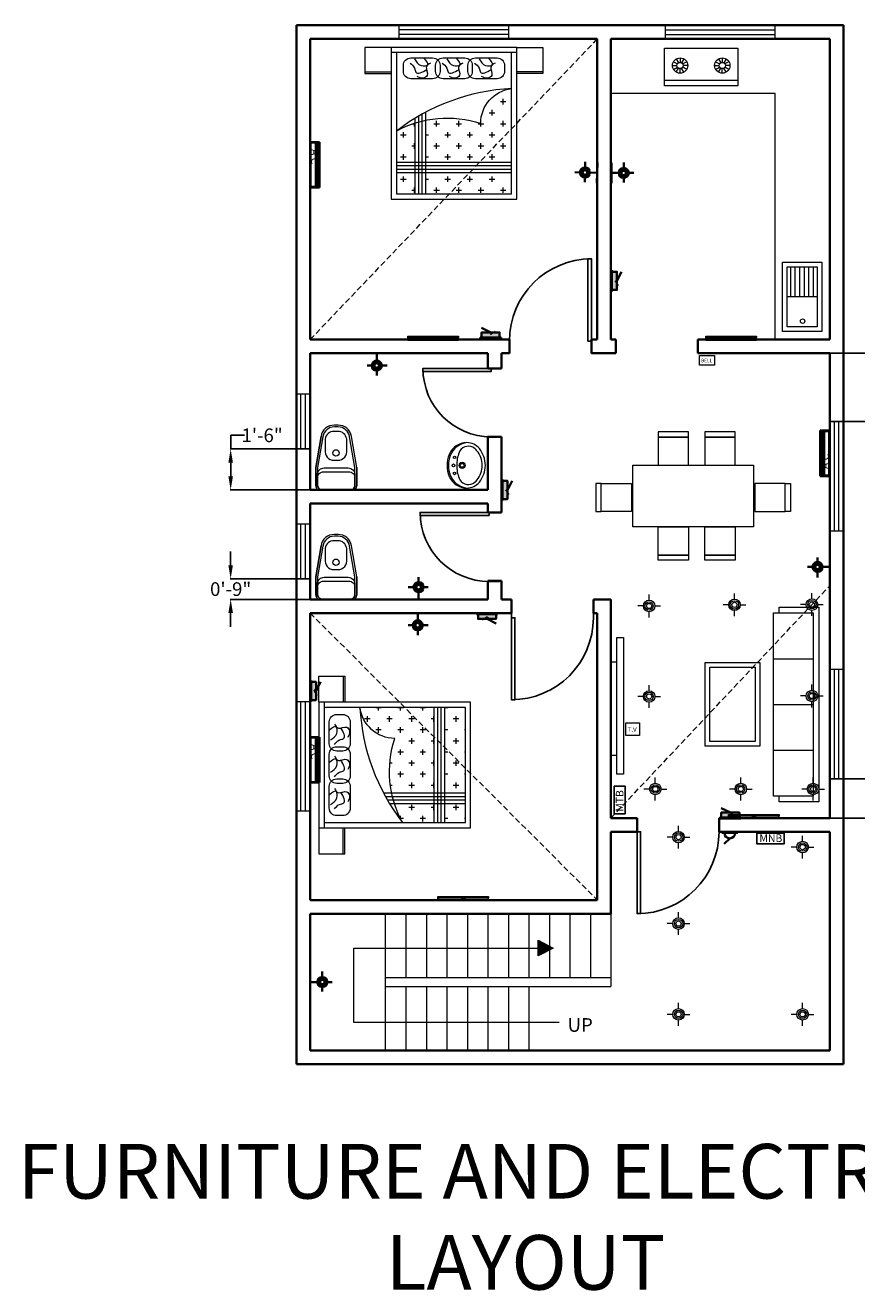
# Model space of a CAD drawing. Units: inches. Extents: x 329 to 1300, y 173 to 760.
# Tile 2 of 3: x 720 to 1085, y 173 to 729. Entities that reach past the tile are written whole.
import ezdxf

# ---------------------------------------------------------------- set-up
doc = ezdxf.new("R2010")
doc.units = ezdxf.units.IN
doc.header["$MEASUREMENT"] = 0
doc.linetypes.add('HIDDEN', pattern=[0.375, 0.25, -0.125])
for name, color, linetype, lineweight in [('A -Elec', 6, 'Continuous', 18), ('A-ANNO-SYMB', 7, 'Continuous', 18), ('A-ANNO-TEXT', 7, 'Continuous', 18), ('A-ANNO-TITL', 1, 'Continuous', 25), ('A-EQPM', 8, 'Continuous', 18), ('A-FLOR-CASE', 163, 'Continuous', 18), ('A-FLOR-FIXT', 163, 'Continuous', 18), ('A-FLOR-STRS', 7, 'Continuous', 18), ('A-FURN', 150, 'Continuous', 5), ('A-GLAZ', 4, 'Continuous', 18), ('A-WALL', 7, 'Continuous', 35), ('DIMENSION', 80, 'Continuous', 13), ('DOOR', 27, 'Continuous', 25), ('E-COMM', 1, 'Continuous', 18), ('E-EQPM-HIDN', 1, 'HIDDEN', 13), ('E-LITE', 6, 'Continuous', 18), ('E-LITE-SWCH', 1, 'Continuous', 18), ('E-POWR-PANL', 1, 'Continuous', 25), ('Elec', 1, 'Continuous', 35), ('FURN', 163, 'Continuous', 5), ('FURNITURE', 163, 'Continuous', 18), ('M-HVAC-EQPM', 1, 'Continuous', 18)]:
    doc.layers.add(name, color=color, linetype=linetype, lineweight=lineweight)
doc.layers.add('A-ANNO-PATT', color=251, linetype='Continuous', lineweight=13, true_color=0x636466)
doc.styles.get("Standard").update_dxf_attribs({"font": 'arial.ttf'})
doc.dimstyles.get("Standard").update_dxf_attribs({"dimtxt": 6, "dimasz": 6, "dimexe": 0.18, "dimexo": 0.0625, "dimgap": 0.09, "dimtad": 0, "dimtih": 1, "dimtoh": 1, "dimdec": 1, "dimzin": 0, "dimdsep": 46, "dimlunit": 3, "dimtxsty": 'Standard', "dimcen": 0.09, "dimadec": 0, "dimazin": 0, "dimtfac": 1, "dimtdec": 1, "dimtofl": 0, "dimtmove": 0, "dimatfit": 3, "dimfxl": 1, "dimtolj": 1, "dimtzin": 0, "dimarcsym": 0})

# ---------------------------------------------------------------- blocks, each defined once
blk = doc.blocks.new('*U2')
for p, q in [((0, 0), (0, -6)), ((40, 0), (40, -6))]:
    blk.add_line(p, q)
blk.add_lwpolyline([(0, 0), (0, 40), (1.75, 40), (1.75, 0)], close=True)
blk.add_arc((0, 0), 40, 0, 90)
blk = doc.blocks.new('TV')
for points in [[(1846.64, 1133.16), (1849.49, 1133.16), (1849.49, 1073.14), (1846.64, 1073.14)], [(1846.64, 1122.37), (1844, 1122.37), (1844, 1081.48), (1846.64, 1081.48)]]:
    blk.add_lwpolyline(points, close=True)
blk = doc.blocks.new('SINK')
for p, q in [((1691.4, 1155.42), (1708.6, 1155.42)), ((1708.6, 1155.42), (1708.6, 1125.07)), ((1693.4, 1140.25), (1706.6, 1140.25)), ((1695.01, 1140.25), (1695.01, 1127.07)), ((1697.01, 1140.25), (1697.01, 1127.07)), ((1699.01, 1140.25), (1699.01, 1127.07)), ((1701.01, 1140.25), (1701.01, 1127.07)), ((1703.01, 1140.25), (1703.01, 1127.07)), ((1705.01, 1140.25), (1705.01, 1127.07))]:
    blk.add_line(p, q)
for points in [[(1691.4, 1155.42), (1708.6, 1155.42), (1708.6, 1125.07), (1691.4, 1125.07)], [(1693.4, 1153.42), (1706.6, 1153.42), (1706.6, 1127.07), (1693.4, 1127.07)]]:
    blk.add_lwpolyline(points, close=True)
blk.add_circle((1699.78, 1150.93), 0.965)
blk = doc.blocks.new('*U16')
blk.add_line((0, 1), (0, -1))
blk = doc.blocks.new('*U17')
at = {"layer": 'FURN', "transparency": 16777216}
for p, rotation in [((1739.06, 1057.24), 90), ((1739.38, 1058.42), 59.99999999999999), ((1739.38, 1056.06), 120), ((1740.24, 1059.29), 30), ((1740.24, 1055.19), 150), ((1741.42, 1054.87), 180), ((1742.61, 1059.29), 330.0000000000001), ((1742.61, 1055.19), 210), ((1743.47, 1058.42), 300), ((1743.47, 1056.06), 240), ((1743.79, 1057.24), 270)]:
    blk.add_blockref('*U16', p, dxfattribs=dict(at, rotation=rotation))
blk.add_blockref('*U16', (1741.42, 1059.61), dxfattribs=at)
blk = doc.blocks.new('*U18')
blk.add_line((0, 1), (0, -1))
blk = doc.blocks.new('*U19')
at = {"layer": 'FURN', "transparency": 16777216}
for p, rotation in [((1739.06, 1057.24), 90), ((1739.38, 1058.42), 59.99999999999999), ((1739.38, 1056.06), 120), ((1740.24, 1059.29), 30), ((1740.24, 1055.19), 150), ((1741.42, 1054.87), 180), ((1742.61, 1059.29), 330.0000000000001), ((1742.61, 1055.19), 210), ((1743.47, 1058.42), 300), ((1743.47, 1056.06), 240), ((1743.79, 1057.24), 270)]:
    blk.add_blockref('*U18', p, dxfattribs=dict(at, rotation=rotation))
blk.add_blockref('*U18', (1741.42, 1059.61), dxfattribs=at)
blk = doc.blocks.new('GAS')
at = {"layer": 'FURN'}
blk.add_line((1734.58, 1063.74), (1766.85, 1063.74), dxfattribs=at)
blk.add_lwpolyline([(1734.58, 1066.15), (1766.85, 1066.15), (1766.85, 1049.65), (1734.58, 1049.65)], close=True, dxfattribs=at)
for centre, radius in [((1741.42, 1057.24), 3.37), ((1741.42, 1057.24), 1.37), ((1759.93, 1057.24), 3.37), ((1759.93, 1057.24), 1.37)]:
    blk.add_circle(centre, radius, dxfattribs=at)
for name, p in [('*U17', (0, 0)), ('*U19', (18.51, 0))]:
    blk.add_blockref(name, p, dxfattribs=at)
blk = doc.blocks.new('bed 1')
at = {"layer": 'FURN'}
h = blk.add_hatch(dxfattribs=at)
h.set_pattern_fill('CROSS', color=256, style=0)
h.set_pattern_definition([(0, (0, 0), (6.35, 6.35), [3.175, -9.525]), (90, (1.5875, -1.5875), (-6.35, 6.35), [3.175, -9.525])])
h.paths.add_polyline_path([(1334.16, -843.32, 0.37496), (1316.43, -863.27, 0.131129), (1284.95, -861.51), (1284.95, -885.72), (1334.16, -885.72)])
h.paths.add_polyline_path([(1278.95, -863.08, 0.048033), (1268.16, -867.67), (1268.16, -885.72), (1278.95, -885.72)])
h.paths.add_polyline_path([(1278.95, -891.72), (1268.16, -891.72), (1268.16, -903.72), (1278.95, -903.72)])
h.paths.add_polyline_path([(1334.16, -891.72), (1284.95, -891.72), (1284.95, -903.72), (1334.16, -903.72)])
for p, q in [((1265.16, -819.72), (1250.16, -819.72)), ((1250.16, -819.72), (1250.16, -834.72)), ((1337.16, -819.72), (1265.16, -819.72)), ((1265.16, -819.72), (1265.16, -906.72)), ((1337.16, -906.72), (1337.16, -819.72)), ((1337.16, -819.72), (1352.16, -819.72)), ((1352.16, -819.72), (1352.16, -834.72)), ((1337.16, -822.72), (1265.16, -822.72)), ((1268.16, -822.72), (1268.16, -903.72)), ((1334.16, -903.72), (1334.16, -822.72)), ((1250.16, -833.72), (1265.16, -833.72)), ((1352.16, -833.72), (1337.16, -833.72)), ((1250.16, -834.72), (1265.16, -834.72)), ((1352.16, -834.72), (1337.16, -834.72)), ((1278.95, -903.72), (1278.95, -860.29)), ((1280.95, -903.72), (1280.95, -859.11)), ((1282.95, -903.72), (1282.95, -857.98)), ((1284.95, -903.72), (1284.95, -856.89)), ((1334.16, -885.72), (1268.16, -885.72)), ((1334.16, -887.72), (1268.16, -887.72)), ((1334.16, -889.72), (1268.16, -889.72)), ((1334.16, -891.72), (1268.16, -891.72)), ((1265.16, -906.72), (1337.16, -906.72)), ((1268.16, -903.72), (1334.16, -903.72))]:
    blk.add_line(p, q, dxfattribs=at)
for points in [[(1288.91, -837.72), (1276.42, -837.72, -0.414214), (1272.16, -833.47), (1272.16, -829.98, -0.414214), (1276.42, -825.72), (1288.91, -825.72, -0.414214), (1293.16, -829.98), (1293.16, -833.47, -0.414214)], [(1307.41, -837.72), (1294.92, -837.72, -0.414214), (1290.66, -833.47), (1290.66, -829.98, -0.414214), (1294.92, -825.72), (1307.41, -825.72, -0.414214), (1311.66, -829.98), (1311.66, -833.47, -0.414214)], [(1325.91, -837.72), (1313.42, -837.72, -0.414214), (1309.16, -833.47), (1309.16, -829.98, -0.414214), (1313.42, -825.72), (1325.91, -825.72, -0.414214), (1330.16, -829.98), (1330.16, -833.47, -0.414214)], [(1334.16, -843.32, 0.151933), (1268.16, -867.67), (1268.16, -867.67, -0.20661), (1316.43, -863.27), (1316.43, -863.27, -0.37496)]]:
    blk.add_lwpolyline(points, format="xyb", close=True, dxfattribs=at)
for points, knots in [([(1278.62, -826.37), (1279.52, -827.92), (1281.07, -830.61), (1287.77, -830.3), (1285.41, -827.44), (1284.17, -825.93)], [0, 0, 0, 0, 4.23607, 7.317462, 10.761159, 10.761159, 10.761159, 10.761159]), ([(1297.12, -826.37), (1298.02, -827.92), (1299.57, -830.61), (1306.27, -830.3), (1303.91, -827.44), (1302.67, -825.93)], [0, 0, 0, 0, 4.23607, 7.317462, 10.761159, 10.761159, 10.761159, 10.761159]), ([(1315.62, -826.37), (1316.52, -827.92), (1318.07, -830.61), (1324.77, -830.3), (1322.41, -827.44), (1321.17, -825.93)], [0, 0, 0, 0, 4.23607, 7.317462, 10.761159, 10.761159, 10.761159, 10.761159]), ([(1275.98, -828.74), (1277, -829.54), (1278.71, -830.85), (1279.22, -835.95), (1282.92, -833.91), (1285.58, -832.44)], [0, 0, 0, 0, 3.079719, 5.108686, 10.317752, 10.317752, 10.317752, 10.317752]), ([(1287.7, -828.74), (1286.63, -829.38), (1283.96, -830.98), (1287.28, -835.52), (1283.18, -838.02), (1281.17, -836.99), (1280.03, -836.4)], [0, 0, 0, 0, 2.624379, 6.568207, 8.823918, 11.783788, 11.783788, 11.783788, 11.783788]), ([(1294.48, -828.74), (1295.5, -829.54), (1297.21, -830.85), (1297.72, -835.95), (1301.42, -833.91), (1304.08, -832.44)], [0, 0, 0, 0, 3.079719, 5.108686, 10.317752, 10.317752, 10.317752, 10.317752]), ([(1306.2, -828.74), (1305.13, -829.38), (1302.46, -830.98), (1305.78, -835.52), (1301.68, -838.02), (1299.67, -836.99), (1298.53, -836.4)], [0, 0, 0, 0, 2.624379, 6.568207, 8.823918, 11.783788, 11.783788, 11.783788, 11.783788]), ([(1312.98, -828.74), (1314, -829.54), (1315.71, -830.85), (1316.22, -835.95), (1319.92, -833.91), (1322.58, -832.44)], [0, 0, 0, 0, 3.079719, 5.108686, 10.317752, 10.317752, 10.317752, 10.317752]), ([(1324.7, -828.74), (1323.63, -829.38), (1320.96, -830.98), (1324.28, -835.52), (1320.18, -838.02), (1318.17, -836.99), (1317.03, -836.4)], [0, 0, 0, 0, 2.624379, 6.568207, 8.823918, 11.783788, 11.783788, 11.783788, 11.783788])]:
    blk.add_open_spline(points, degree=3, knots=knots, dxfattribs=at)
blk = doc.blocks.new('WC')
at = {"layer": 'A-FURN'}
for p, q in [((171114.18, -56009.21), (171100.52, -56011.54)), ((171114.18, -56009.21), (171122.29, -56009.21)), ((171124.07, -56010.99), (171124.07, -56025.42)), ((171095.59, -56017.39), (171095.59, -56019.02)), ((171114.18, -56027.21), (171100.52, -56024.87)), ((171122.29, -56027.21), (171114.18, -56027.21))]:
    blk.add_line(p, q, dxfattribs=at)
for points in [[(171114.18, -56027.21), (171122.29, -56027.21, 0.414214), (171124.07, -56025.42), (171124.07, -56010.99, 0.414214), (171122.29, -56009.21), (171114.18, -56009.21), (171100.52, -56011.54, 0.365402), (171095.59, -56017.39), (171095.59, -56019.02, 0.365402), (171100.52, -56024.87)], [(171114.25, -56026.41), (171121.5, -56026.41, 0.361508), (171124.07, -56024.7), (171124.07, -56011.71, 0.375474), (171121.68, -56010), (171114.25, -56010), (171100.66, -56012.32, 0.365402), (171096.38, -56017.39), (171096.38, -56019.02, 0.365402), (171100.66, -56024.09)], [(171124.07, -56011.71), (171124.07, -56024.7, -0.361508), (171121.5, -56026.41), (171117.23, -56026.41, -0.430105), (171114.38, -56023.46), (171114.38, -56012.95, -0.411531), (171117.23, -56010), (171121.68, -56010, -0.375474)], [(171124.07, -56011.71), (171124.07, -56024.7, -0.361508), (171121.5, -56026.41), (171118.83, -56026.41, -0.480412), (171116.16, -56023.63), (171116.16, -56012.78, -0.482705), (171118.83, -56010), (171121.68, -56010, -0.375474)], [(171106.42, -56023.02, 0.46477), (171111.04, -56019.12), (171111.04, -56017.49, 0.46477), (171106.42, -56013.59), (171101.64, -56013.59, 0.365402), (171098.35, -56017.49), (171098.35, -56019.12, 0.365402), (171101.64, -56023.02)], [(171107.8, -56016.9, -1), (171107.8, -56019.71, -1)]]:
    blk.add_lwpolyline(points, format="xyb", close=True, dxfattribs=at)
for centre, radius, start, end in [((171122.29, -56010.99), 1.78, 0.0002, 90.0002), ((171101.52, -56017.39), 5.93, 99.7106, 180.0002), ((171101.52, -56019.02), 5.93, 180.0002, 260.2897), ((171122.29, -56025.42), 1.78, 270.0002, 0.0002)]:
    blk.add_arc(centre, radius, start, end, dxfattribs=at)
blk = doc.blocks.new('Basin')
at = {"layer": 'A-FURN'}
for centre, radius in [((171010.96, -56068.51), 0.593), ((171010.45, -56072.47), 0.692), ((171014.68, -56072.47), 1.48), ((171014.68, -56072.47), 0.91), ((171010.96, -56076.42), 0.593)]:
    blk.add_circle(centre, radius, dxfattribs=at)
for centre, radius, start, end in [((171016.96, -56070.69), 9.3, 90, 157.28559), ((171018.29, -56071.51), 10.2, 100.99675, 157.82074), ((171016.96, -56069.3), 7.91, 39.08291, 90), ((171021.21, -56072.47), 13.91, 157.28559, 180), ((171021.21, -56072.47), 13.27, 158.74675, 180), ((171018.29, -56073.43), 10.2, 262.50469, 262.50469), ((171029.84, -56072.47), 17.8, 159.64154, 180), ((171017.65, -56067.95), 4.81, 62.93101, 159.64154), ((171016.96, -56069.3), 6.33, 39.08291, 62.931), ((171013.06, -56072.47), 11.35, 0, 39.08291), ((171013.06, -56072.47), 12.93, 0, 39.08291), ((171021.21, -56072.47), 13.91, 180, 202.71441), ((171021.21, -56072.47), 13.27, 180, 201.25325), ((171029.84, -56072.47), 17.8, 180, 200.35846), ((171013.06, -56072.47), 11.35, 320.91709, 0), ((171013.06, -56072.47), 12.93, 320.91709, 0), ((171016.96, -56074.25), 9.3, 202.71441, 270), ((171018.29, -56073.43), 10.2, 202.17926, 259.00325), ((171017.65, -56076.99), 4.81, 200.35846, 297.06899), ((171016.96, -56075.63), 6.33, 297.069, 320.91709), ((171016.96, -56075.63), 7.91, 270, 320.91709)]:
    blk.add_arc(centre, radius, start, end, dxfattribs=at)
blk = doc.blocks.new('S')
at = {"layer": 'FURN'}
for p, q in [((1046.36, 480.08), (1063.8, 480.08)), ((1046.36, 459.98), (1063.8, 459.98)), ((1046.36, 439.88), (1063.8, 439.88))]:
    blk.add_line(p, q, dxfattribs=at)
blk.add_lwpolyline([(1063.8, 500.18), (1063.8, 419.78), (1046.36, 419.78), (1046.36, 500.18)], close=True, dxfattribs=at)
blk.add_lwpolyline([(1048.87, 500.18), (1048.87, 502.69), (1066.31, 502.69), (1066.31, 417.27), (1048.87, 417.27), (1048.87, 419.78)], dxfattribs=at)
blk = doc.blocks.new('splight')
at = {"layer": 'Elec'}
for p, q in [((4618.17, 527.16), (4627.57, 527.16)), ((4622.87, 527.16), (4622.87, 523.87)), ((4620.58, 521.58), (4618.05, 521.58)), ((4625.16, 521.58), (4627.23, 521.58)), ((4622.87, 519.28), (4622.87, 517.03))]:
    blk.add_line(p, q, dxfattribs=at)
for radius in [2.29, 1.67, 1.04]:
    blk.add_circle((4622.87, 521.58), radius, dxfattribs=at)
blk = doc.blocks.new('tube')
at = {"layer": 'A -Elec'}
for p, q in [((4592.6, 556.8), (4641.6, 556.8)), ((4592.6, 555.3), (4592.6, 556.8)), ((4592.6, 552.8), (4592.6, 555.3)), ((4592.6, 552.8), (4641.6, 552.8)), ((4593.1, 555.3), (4593.1, 556.8)), ((4593.1, 556.3), (4593.4, 556.3)), ((4593.1, 556.2), (4593.4, 556.2)), ((4593.1, 555.8), (4593.4, 555.8)), ((4593.1, 555.7), (4593.4, 555.7)), ((4641.1, 555.3), (4593.1, 555.3)), ((4593.1, 555.3), (4593.1, 553.3)), ((4593.1, 553.3), (4593.1, 555.3)), ((4593.1, 553.3), (4641.6, 553.3)), ((4593.4, 555.3), (4593.4, 556.8)), ((4593.4, 556.5), (4640.8, 556.5)), ((4593.4, 556.3), (4640.8, 556.3)), ((4593.4, 556), (4640.8, 556)), ((4593.4, 555.8), (4640.8, 555.8)), ((4593.4, 555.5), (4640.8, 555.5)), ((4640.8, 555.3), (4640.8, 556.8)), ((4640.8, 556.3), (4641.1, 556.3)), ((4640.8, 556.2), (4641.1, 556.2)), ((4640.8, 555.8), (4641.1, 555.8)), ((4640.8, 555.7), (4641.1, 555.7)), ((4641.1, 556.8), (4641.1, 555.3)), ((4641.1, 555.3), (4641.1, 556.8)), ((4641.1, 553.3), (4641.1, 555.3)), ((4641.6, 556.8), (4641.6, 555.3)), ((4641.6, 552.8), (4641.6, 555.3))]:
    blk.add_line(p, q, dxfattribs=at)
for points in [[(4615.6, 553.3), (4619.1, 553.3), (4619.1, 554.3), (4615.6, 554.3)], [(4619.1, 553.8), (4619.1, 553.8), (4619.1, 553.8), (4619.1, 553.8)], [(4619.1, 553.8), (4619.8, 553.8), (4619.8, 553.3), (4619.1, 553.3)]]:
    blk.add_lwpolyline(points, close=True, dxfattribs=at)
blk = doc.blocks.new('CIELING')
at = {"layer": 'A -Elec'}
for p, q in [((1070.87, -8395.66), (1070.87, -8391.49)), ((1066.61, -8399.91), (1062.44, -8399.91)), ((1075.13, -8399.91), (1079.29, -8399.91)), ((1070.87, -8408.34), (1070.87, -8404.17))]:
    blk.add_line(p, q, dxfattribs=at)
for radius in [4.26, 3.1, 1.94]:
    blk.add_circle((1070.87, -8399.91), radius, dxfattribs=at)
blk = doc.blocks.new('ac')
at = {"layer": 'Elec'}
for p, q in [((12718.3, -53.8), (12674.4, -53.8)), ((12674.4, -63), (12674.4, -53.8)), ((12674.9, -57.5), (12717.8, -57.5)), ((12675.8, -57.5), (12675.8, -53.8)), ((12717, -54.9), (12675.8, -54.9)), ((12717, -56.2), (12675.8, -56.2)), ((12717, -57.5), (12717, -53.8)), ((12718.3, -63), (12718.3, -53.8)), ((12718.3, -63), (12674.4, -63))]:
    blk.add_line(p, q, dxfattribs=at)
at = {"layer": 'Elec', "ltscale": 0.1}
for p, q in [((12674.9, -61.5), (12674.9, -53.8)), ((12717, -54.4), (12675.8, -54.4)), ((12717, -55.7), (12675.8, -55.7)), ((12717, -56.8), (12675.8, -56.8)), ((12717.8, -61.5), (12717.8, -53.8)), ((12716.8, -62.5), (12675.9, -62.5))]:
    blk.add_line(p, q, dxfattribs=at)
at = {"layer": 'Elec'}
for centre, start, end in [((12675.9, -61.5), 180, 270), ((12716.8, -61.5), 270, 0)]:
    blk.add_arc(centre, 1, start, end, dxfattribs=at)
blk = doc.blocks.new('BELL SWITCH')
at = {"layer": 'Elec'}
for p, q in [((4981.81, 3401.31), (4981.81, 3402.27)), ((4981.81, 3402.27), (4993.57, 3402.27)), ((4993.57, 3401.31), (4981.81, 3401.31)), ((4987.69, 3397.36), (4983.52, 3393.3)), ((4993.57, 3402.27), (4993.57, 3401.31))]:
    blk.add_line(p, q, dxfattribs=at)
blk.add_arc((4987.69, 3401.31), 3.95, 180, 0, dxfattribs=at)
blk = doc.blocks.new('WIN-W1-48IN')
for p, q in [((0, 0), (0, 6)), ((48, 0), (48, 6)), ((0, 4), (48, 4)), ((0, 2), (48, 2))]:
    blk.add_line(p, q)
blk = doc.blocks.new('VENT-V0-24IN')
for p, q in [((6, 24), (0, 24)), ((2, 0), (2, 24)), ((4, 0), (4, 24)), ((6, 0), (0, 0))]:
    blk.add_line(p, q)
blk = doc.blocks.new('CHAIR-DINING-SIDE')
for points in [[(0, 12.34), (13.32, 12.34), (13.32, 14.61), (0, 14.61)], [(0, 0), (13.32, 0), (13.32, 12.34), (0, 12.34)]]:
    blk.add_lwpolyline(points, close=True)
blk = doc.blocks.new('CHAIR-DINING-END')
for points in [[(2.35, 12.34), (0, 12.34), (0, 0), (2.35, 0)], [(2.35, 12.34), (15.66, 12.34), (15.66, 0), (2.35, 0)]]:
    blk.add_lwpolyline(points, close=True)
blk = doc.blocks.new('elec box')
at = {"layer": 'Elec'}
blk.add_hatch(color=256, dxfattribs=at).paths.add_polyline_path([(3828.2, 599.3), (3828.2, 594.8), (3844.7, 594.8), (3844.7, 599.3)])
for p, q in [((3836.5, 599.3), (3828.1, 603.5)), ((3846.1, 594.8), (3826.8, 594.8)), ((3826.8, 594.8), (3826.8, 593.9)), ((3826.8, 593.9), (3846.1, 593.9)), ((3846.1, 593.9), (3846.1, 594.8))]:
    blk.add_line(p, q, dxfattribs=at)
blk.add_lwpolyline([(3828.2, 594.8), (3828.2, 599.3), (3844.7, 599.3), (3844.7, 594.8), (3828.2, 594.8)], dxfattribs=at)
blk = doc.blocks.new('SWITCHBOARD-1WAY')
blk.add_line((4.63, 1.73), (6.64, 3.12))
at = {"xscale": 0.480395109260985, "yscale": 0.480395109260985, "zscale": 0.480395109260985}
blk.add_blockref('elec box', (-1838.39, -285.3), dxfattribs=at)
blk = doc.blocks.new('SWITCHBOARD-2WAY')
for q in [(2.61, 1.47), (6.62, 1.46)]:
    blk.add_line((4.62, 2.87), q)
at = {"xscale": 0.480395109260985, "yscale": 0.480395109260985, "zscale": 0.480395109260985, "rotation": 180}
blk.add_blockref('elec box', (1847.65, 289.9), dxfattribs=at)
blk = doc.blocks.new('BOARD-MAIN')
blk.add_lwpolyline([(0, 4.7), (12.06, 4.7), (12.06, 0), (0, 0)], close=True)
blk.add_text('MNB', height=3.363).set_placement((1.14, 0.8))
blk = doc.blocks.new('BOARD-METER')
blk.add_lwpolyline([(0, 4.7), (12.06, 4.7), (12.06, 0), (0, 0)], close=True)
blk.add_text('MTB', height=3.363).set_placement((0.87, 0.69))
blk = doc.blocks.new('BELL-POINT')
blk.add_lwpolyline([(0, 4.27), (6.56, 4.27), (6.56, 0), (0, 0)], close=True)
at = {"insert": (0.64, 2.8), "char_height": 1.537, "attachment_point": 1}
blk.add_mtext('BELL', dxfattribs=at)
blk = doc.blocks.new('TV-POINT')
blk.add_lwpolyline([(0, 5.57), (6.1, 5.57), (6.1, 0), (0, 0)], close=True)
at = {"transparency": 33554676}
blk.add_lwpolyline([(0, 5.57), (6.1, 5.57), (6.1, 0), (0, 0)], close=True, dxfattribs=at)
at = {"insert": (0.84, 3.65), "char_height": 2.003, "attachment_point": 1}
blk.add_mtext('T.V ', dxfattribs=at)
at = {"transparency": 33554676, "insert": (0.84, 3.65), "char_height": 2.003, "attachment_point": 1}
blk.add_mtext('T.V ', dxfattribs=at)
blk = doc.blocks.new('*D53')
at = {"layer": 'Defpoints', "color": 0, "transparency": 16777216}
for p in [(1072.98, 397.84), (1107.83, 397.84), (1072.98, 380.62)]:
    blk.add_point(p, dxfattribs=at)
at = {"layer": 'DIMENSION', "color": 0, "lineweight": -2, "transparency": 16777216}
for p, q in [((1107.83, 397.84), (1107.83, 403.84)), ((1107.83, 403.84), (1113.83, 403.84)), ((1073.04, 397.84), (1108.01, 397.84)), ((1107.83, 386.62), (1107.83, 391.84)), ((1073.04, 380.62), (1108.01, 380.62))]:
    blk.add_line(p, q, dxfattribs=at)
at = {"layer": 'DIMENSION', "color": 0, "transparency": 16777216}
for points in [[(1106.83, 391.84), (1108.83, 391.84), (1107.83, 397.84)], [(1106.83, 386.62), (1108.83, 386.62), (1107.83, 380.62)]]:
    blk.add_solid(points, dxfattribs=at)
at = {"layer": 'DIMENSION', "color": 0, "transparency": 16777216, "insert": (1121.61, 403.84), "char_height": 6, "attachment_point": 5}
blk.add_mtext('\\A1;1\'-5"', dxfattribs=at)
blk = doc.blocks.new('*D56')
at = {"layer": 'Defpoints', "color": 0, "transparency": 16777216}
for p in [(810.13, 542.62), (844.98, 542.62), (844.98, 524.62)]:
    blk.add_point(p, dxfattribs=at)
at = {"layer": 'DIMENSION', "color": 0, "lineweight": -2, "transparency": 16777216}
for p, q in [((810.13, 542.62), (810.13, 548.62)), ((810.13, 548.62), (816.13, 548.62)), ((844.91, 542.62), (809.95, 542.62)), ((810.13, 530.62), (810.13, 536.62)), ((844.91, 524.62), (809.95, 524.62))]:
    blk.add_line(p, q, dxfattribs=at)
at = {"layer": 'DIMENSION', "color": 0, "transparency": 16777216}
for points in [[(809.13, 536.62), (811.13, 536.62), (810.13, 542.62)], [(809.13, 530.62), (811.13, 530.62), (810.13, 524.62)]]:
    blk.add_solid(points, dxfattribs=at)
at = {"layer": 'DIMENSION', "color": 0, "transparency": 16777216, "insert": (823.91, 548.62), "char_height": 6, "attachment_point": 5}
blk.add_mtext('\\A1;1\'-6"', dxfattribs=at)
blk = doc.blocks.new('*D57')
at = {"layer": 'Defpoints', "color": 0, "transparency": 16777216}
for p in [(810.125195, 485.617223), (844.975195, 485.617223), (844.975195, 476.617223)]:
    blk.add_point(p, dxfattribs=at)
at = {"layer": 'DIMENSION', "color": 0, "lineweight": -2, "transparency": 16777216}
for p, q in [((810.125195, 491.617223), (810.125195, 497.617223)), ((844.912695, 485.617223), (809.945195, 485.617223)), ((844.912695, 476.617223), (809.945195, 476.617223)), ((810.125195, 470.617223), (810.125195, 464.617223))]:
    blk.add_line(p, q, dxfattribs=at)
at = {"layer": 'DIMENSION', "color": 0, "transparency": 16777216}
for points in [[(809.125195, 491.617223), (811.125195, 491.617223), (810.125195, 485.617223)], [(809.125195, 470.617223), (811.125195, 470.617223), (810.125195, 476.617223)]]:
    blk.add_solid(points, dxfattribs=at)
at = {"layer": 'DIMENSION', "color": 0, "transparency": 16777216, "insert": (810.125195, 481.117223), "char_height": 6, "attachment_point": 5}
blk.add_mtext('\\A1;0\'-9"', dxfattribs=at)
blk = doc.blocks.new('*D58')
at = {"layer": 'Defpoints', "color": 0, "transparency": 16777216}
for p in [(1072.98, 584.62), (1107.83, 584.62), (1072.98, 554.62)]:
    blk.add_point(p, dxfattribs=at)
at = {"layer": 'DIMENSION', "color": 0, "lineweight": -2, "transparency": 16777216}
for p, q in [((1073.04, 584.62), (1108.01, 584.62)), ((1107.83, 578.62), (1107.83, 572.77)), ((1107.83, 560.62), (1107.83, 566.46)), ((1073.04, 554.62), (1108.01, 554.62))]:
    blk.add_line(p, q, dxfattribs=at)
at = {"layer": 'DIMENSION', "color": 0, "transparency": 16777216}
for points in [[(1106.83, 578.62), (1108.83, 578.62), (1107.83, 584.62)], [(1106.83, 560.62), (1108.83, 560.62), (1107.83, 554.62)]]:
    blk.add_solid(points, dxfattribs=at)
at = {"layer": 'DIMENSION', "color": 0, "transparency": 16777216, "insert": (1107.83, 569.62), "char_height": 6, "attachment_point": 5}
blk.add_mtext('\\A1;2\'-6"', dxfattribs=at)

msp = doc.modelspace()

# ---------------------------------------------------------------- hatches: boundary and pattern name
at = {"layer": 'A-ANNO-PATT'}
h = msp.add_hatch(dxfattribs=at)
h.set_pattern_fill('ANSI31', color=256)
h.set_pattern_definition([(45, (472.30385, 0), (-0.088388348, 0.088388348), [])])
h.paths.add_polyline_path([(949.98, 324.36), (945.1, 326.94), (945.1, 323.48), (945.1, 320.13), (949.98, 322.63)])
h.paths.add_polyline_path([(951.64, 323.48), (949.98, 324.36), (949.98, 322.63)])
h = msp.add_hatch(color=256, dxfattribs=at)
h.dxf.hatch_style = 1
h.paths.add_polyline_path([(949.98, 324.36), (945.1, 326.94), (945.1, 323.48), (945.1, 320.13), (949.98, 322.63)])
h.paths.add_polyline_path([(949.98, 324.36), (949.98, 322.63), (951.64, 323.48)])

# ---------------------------------------------------------------- linework, layer by layer
at = {"layer": 'A-ANNO-SYMB'}
for p, q in [((864.14, 290.84), (864.14, 323.48)), ((864.14, 323.48), (945.1, 323.48)), ((945.1, 323.48), (945.1, 326.94)), ((945.1, 326.94), (951.64, 323.48)), ((951.64, 323.48), (945.1, 320.13)), ((945.1, 320.13), (945.1, 323.48)), ((954.29, 290.84), (864.14, 290.84))]:
    msp.add_line(p, q, dxfattribs=at)
at = {"layer": 'A-FLOR-CASE'}
for p, q in [((1048.98, 698.62), (976.98, 698.62)), ((1048.98, 590.62), (1048.98, 698.62))]:
    msp.add_line(p, q, dxfattribs=at)
at = {"layer": 'A-FLOR-STRS'}
for p, q in [((877.98, 338.62), (877.98, 278.62)), ((886.98, 338.62), (886.98, 310.62)), ((895.98, 338.62), (895.98, 310.62)), ((904.98, 338.62), (904.98, 310.62)), ((913.98, 338.62), (913.98, 310.62)), ((922.98, 338.62), (922.98, 310.62)), ((931.98, 338.62), (931.98, 310.62)), ((940.98, 338.62), (940.98, 310.62)), ((949.98, 338.62), (949.98, 324.36)), ((958.98, 338.62), (958.98, 310.62)), ((967.98, 338.62), (967.98, 310.62)), ((976.98, 338.62), (976.98, 306.62)), ((949.98, 322.63), (949.98, 310.62)), ((877.98, 310.62), (976.98, 310.62)), ((877.98, 306.62), (976.98, 306.62)), ((886.98, 306.62), (886.98, 278.62)), ((895.98, 306.62), (895.98, 278.62)), ((904.98, 306.62), (904.98, 278.62)), ((913.98, 306.62), (913.98, 278.62)), ((922.98, 306.62), (922.98, 278.62)), ((931.98, 306.62), (931.98, 278.62)), ((940.98, 306.62), (940.98, 278.62))]:
    msp.add_line(p, q, dxfattribs=at)
at = {"layer": 'A-WALL'}
for p, q in [((1078.98, 728.62), (838.98, 728.62)), ((838.98, 728.62), (838.98, 272.62)), ((1078.98, 272.62), (1078.98, 728.62)), ((970.98, 722.62), (844.98, 722.62)), ((844.98, 722.62), (844.98, 590.62)), ((970.98, 722.62), (970.98, 590.62)), ((1072.98, 722.62), (976.98, 722.62)), ((976.98, 722.62), (976.98, 590.62)), ((1072.98, 590.62), (1072.98, 722.62)), ((932.45, 590.62), (844.98, 590.62)), ((932.45, 590.62), (932.45, 584.62)), ((970.98, 590.62), (968.45, 590.62)), ((968.45, 590.62), (968.45, 584.62)), ((979.12, 590.62), (976.98, 590.62)), ((979.12, 590.62), (979.12, 584.62)), ((1072.98, 590.62), (1015.12, 590.62)), ((1015.12, 590.62), (1015.12, 584.62)), ((922.98, 584.62), (844.98, 584.62)), ((844.98, 584.62), (844.98, 524.62)), ((922.98, 584.62), (922.98, 577.98)), ((932.45, 584.62), (928.98, 584.62)), ((928.98, 584.62), (928.98, 577.98)), ((976.98, 584.62), (968.45, 584.62)), ((979.12, 584.62), (976.98, 584.62)), ((1072.98, 584.62), (1015.12, 584.62)), ((1072.98, 380.62), (1072.98, 584.62)), ((922.98, 577.98), (928.98, 577.98)), ((922.98, 547.98), (922.98, 524.62)), ((922.98, 547.98), (928.98, 547.98)), ((928.98, 547.98), (928.98, 524.62)), ((922.98, 524.62), (844.98, 524.62)), ((928.98, 524.62), (928.98, 514.8)), ((922.98, 518.62), (844.98, 518.62)), ((844.98, 518.62), (844.98, 476.62)), ((922.98, 518.62), (922.98, 514.8)), ((922.98, 514.8), (928.98, 514.8)), ((922.98, 484.8), (922.98, 476.62)), ((922.98, 484.8), (928.98, 484.8)), ((928.98, 484.8), (928.98, 476.62)), ((922.98, 476.62), (844.98, 476.62)), ((933.28, 476.62), (928.98, 476.62)), ((933.28, 470.62), (933.28, 476.62)), ((976.98, 476.62), (969.28, 476.62)), ((969.28, 470.62), (969.28, 476.62)), ((976.98, 476.62), (976.98, 380.62)), ((933.28, 470.62), (844.98, 470.62)), ((844.98, 470.62), (844.98, 344.62)), ((970.98, 470.62), (969.28, 470.62)), ((970.98, 470.62), (970.98, 344.62)), ((988.41, 380.62), (976.98, 380.62)), ((988.41, 374.62), (988.41, 380.62)), ((1072.98, 380.62), (1024.41, 380.62)), ((1024.41, 374.62), (1024.41, 380.62)), ((988.41, 374.62), (976.98, 374.62)), ((976.98, 374.62), (976.98, 338.62)), ((1072.98, 374.62), (1024.41, 374.62)), ((1072.98, 278.62), (1072.98, 374.62)), ((970.98, 344.62), (844.98, 344.62)), ((976.98, 338.62), (844.98, 338.62)), ((844.98, 338.62), (844.98, 278.62)), ((844.98, 278.62), (1072.98, 278.62)), ((838.98, 272.62), (1078.98, 272.62))]:
    msp.add_line(p, q, dxfattribs=at)
at = {"layer": 'E-EQPM-HIDN', "ltscale": 10}
for p, q in [((844.98, 590.62), (970.98, 722.62)), ((976.98, 380.62), (1072.98, 482.62)), ((844.98, 470.62), (970.98, 344.62))]:
    msp.add_line(p, q, dxfattribs=at)
at = {"layer": 'FURNITURE'}
for points in [[(986.56, 535.48), (1039.58, 535.48), (1039.58, 508.38), (986.56, 508.38)], [(1042.27, 412.16), (1018.34, 412.16), (1018.34, 448.86), (1042.27, 448.86)], [(1040.27, 414.16), (1020.34, 414.16), (1020.34, 446.86), (1040.27, 446.86)]]:
    msp.add_lwpolyline(points, close=True, dxfattribs=at)

# ---------------------------------------------------------------- block references
at = {"layer": 'A-EQPM', "rotation": 179.9999999999993}
msp.add_blockref('GAS', (2767.24, 1768.2), dxfattribs=at)
at = {"layer": 'A-EQPM'}
msp.add_blockref('TV', (-867.02, -673.31), dxfattribs=at)
at = {"layer": 'A-FLOR-FIXT'}
for name, p, rotation in [('SINK', (2760.84, 1749.66), 180), ('WC', (56874.64, 171648.69), 270), ('WC', (56874.64, 171600.69), 270)]:
    msp.add_blockref(name, p, dxfattribs=dict(at, rotation=rotation))
at = {"layer": 'A-FLOR-FIXT', "ltscale": 0.05, "xscale": 0.900000000023283, "yscale": 0.900000000023283, "zscale": 0.900000000023283}
msp.add_blockref('Basin', (-153001.52, 51000.66), dxfattribs=at)
at = {"layer": 'A-GLAZ'}
for p, rotation in [((931.98, 728.62), 180), ((1078.98, 506.62), 90.00000000000003), ((1078.98, 397.84), 90.00000000000003), ((844.98, 383.62), 90.00000000000003)]:
    msp.add_blockref('WIN-W1-48IN', p, dxfattribs=dict(at, rotation=rotation))
for name, p in [('WIN-W1-48IN', (1000.97, 722.62)), ('VENT-V0-24IN', (838.98, 542.62)), ('VENT-V0-24IN', (838.98, 485.62))]:
    msp.add_blockref(name, p, dxfattribs=at)
at = {"layer": 'DOOR', "xscale": -0.9012848244184455, "yscale": 0.9012848244184455, "zscale": 0.9012848244184455}
msp.add_blockref('*U2', (968.45, 590.02), dxfattribs=at)
at = {"layer": 'DOOR'}
for p, xscale, yscale, zscale, rotation in [((924.48, 577.98), -0.7497467609316112, 0.7497467609316112, 0.7497467609316112, 90), ((923.52, 514.8), -0.7577850931716829, 0.7577850931716829, 0.7577850931716829, 90), ((933.28, 468.52), -0.8991931185370194, 0.8991931185370194, 0.8991931185370194, 180), ((988.41, 374.6), -0.8991931185370194, 0.8991931185370194, 0.8991931185370194, 180)]:
    msp.add_blockref('*U2', p, dxfattribs=dict(at, xscale=xscale, yscale=yscale, zscale=zscale, rotation=rotation))
at = {"layer": 'E-COMM'}
for name, p in [('BELL-POINT', (1015.87, 579.45)), ('TV-POINT', (983.45, 416.81))]:
    msp.add_blockref(name, p, dxfattribs=at)
at = {"layer": 'E-COMM', "xscale": 0.6004938865802444, "yscale": 0.6004938865802444, "zscale": 0.6004938865802444}
msp.add_blockref('BELL SWITCH', (-1965.97, -1668.42), dxfattribs=at)
at = {"layer": 'E-LITE', "zscale": 0.9617510087390623}
for p, xscale, yscale, rotation in [((563.71, 5120.16), 0.9617510087435098, 0.9617510087435098, 268.7154029599204), ((1484.2, 5109.84), -0.9617510087435096, 0.9617510087435096, 89.99999999999976), ((5320.26, 77.62), -0.9617510087435096, 0.9617510087435096, 359.9999999999997), ((565.98, -3955.21), -0.9617510087435096, 0.9617510087435096, 269.9999999999998), ((-3553.48, 983.61), -0.9617510087435096, 0.9617510087435096, 180), ((5338.23, -36.38), -0.9617510087435096, 0.9617510087435096, 359.9999999999997), ((1351.97, 4754.67), -0.9617510087435096, 0.9617510087435096, 89.99999999999976)]:
    msp.add_blockref('splight', p, dxfattribs=dict(at, xscale=xscale, yscale=yscale, rotation=rotation))
at = {"layer": 'E-LITE', "transparency": 33554676}
for name, p, xscale, yscale, zscale in [('tube', (-1194.72, 339.73), 0.4534687213066354, 0.4534687213066354, 0.4534687213066354), ('tube', (-1063.95, 339.73), 0.4534687213066354, 0.4534687213066354, 0.4534687213066354), ('CIELING', (358.63, 5455.3), 0.5930528030907906, 0.5930528030907906, 0.5930528030907906), ('CIELING', (396.08, 5455.78), 0.5930528030907906, 0.5930528030907906, 0.5930528030907906), ('CIELING', (430.07, 5455.9), 0.5930528030907906, 0.5930528030907906, 0.5930528030907906), ('CIELING', (358.63, 5415.57), 0.5930528030907906, 0.5930528030907906, 0.5930528030907906), ('CIELING', (430.07, 5415.79), 0.5930528030907906, 0.5930528030907906, 0.5930528030907906), ('CIELING', (361.35, 5374.94), 0.5930528030907906, 0.5930528030907906, 0.5930528030907906), ('CIELING', (398.85, 5374.94), 0.5930528030907906, 0.5930528030907906, 0.5930528030907906), ('CIELING', (430.57, 5374.94), 0.5930528030907906, 0.5930528030907906, 0.5930528030907906), ('tube', (-1054.11, 129.73), 0.4534687213066354, 0.4534687213066354, 0.4534687213066354), ('CIELING', (371.55, 5353.82), 0.5930528030907906, 0.5930528030907906, 0.5930528030907906), ('CIELING', (425.97, 5349.46), 0.5930528030907906, 0.5930528030907906, 0.5930528030907906), ('tube', (-1181.56, 93.73), 0.4534687213066354, 0.4534687213066354, 0.4534687213066354), ('CIELING', (371.55, 5315.86), 0.5930528030907906, 0.5930528030907906, 0.5930528030907906), ('CIELING', (371.55, 5276.02), 0.5930528030907906, 0.5930528030907906, 0.5930528030907906), ('CIELING', (425.97, 5276.02), 0.5930528030907906, 0.5930528030907906, 0.5930528030907906)]:
    msp.add_blockref(name, p, dxfattribs=dict(at, xscale=xscale, yscale=yscale, zscale=zscale))
at = {"layer": 'E-LITE-SWCH'}
for name, p, rotation in [('SWITCHBOARD-1WAY', (976.98, 621.07), 269.9999999999994), ('SWITCHBOARD-1WAY', (928.98, 529.25), 269.9999999999997), ('SWITCHBOARD-2WAY', (849.57, 431.74), 89.99999999999818)]:
    msp.add_blockref(name, p, dxfattribs=dict(at, rotation=rotation))
for name, p in [('SWITCHBOARD-1WAY', (919.56, 591.18)), ('SWITCHBOARD-2WAY', (917.99, 466.02)), ('SWITCHBOARD-1WAY', (1024.72, 380.39))]:
    msp.add_blockref(name, p, dxfattribs=at)
at = {"layer": 'E-POWR-PANL', "rotation": 89.99999999999866}
msp.add_blockref('BOARD-METER', (983.15, 382.53), dxfattribs=at)
at = {"layer": 'E-POWR-PANL'}
msp.add_blockref('BOARD-MAIN', (1040.97, 369.29), dxfattribs=at)
at = {"layer": 'FURNITURE', "xscale": 0.7655046386938622, "yscale": 0.7655046386875327, "zscale": 0.7655046386898116}
msp.add_blockref('bed 1', (-87.95, 1346.42), dxfattribs=at)
at = {"layer": 'FURNITURE'}
for name, p in [('CHAIR-DINING-SIDE', (997.7, 535.48)), ('CHAIR-DINING-SIDE', (1018.19, 535.48)), ('CHAIR-DINING-END', (970.38, 515.14)), ('S', (1.86, -29.54))]:
    msp.add_blockref(name, p, dxfattribs=at)
at = {"layer": 'FURNITURE', "extrusion": (0, 0, -1), "zscale": -1}
msp.add_blockref('CHAIR-DINING-END', (-1055.75, 515.14), dxfattribs=at)
at = {"layer": 'FURNITURE', "extrusion": (0, 0, -1), "zscale": -1, "rotation": 180}
for p in [(-997.7, 508.38), (-1018.19, 508.38)]:
    msp.add_blockref('CHAIR-DINING-SIDE', p, dxfattribs=at)
at = {"layer": 'FURNITURE', "xscale": 0.7655046386938622, "yscale": 0.7655046386875327, "zscale": 0.7655046386898116, "rotation": 90}
msp.add_blockref('bed 1', (221.29, -592.17), dxfattribs=at)
at = {"layer": 'M-HVAC-EQPM', "xscale": 0.4550488862921059, "yscale": 0.4550488862921059, "zscale": 0.4550488862921059}
for p, rotation in [((873.65, 6444.86), 270), ((1044.3, -5236.76), 90), ((873.65, 6183.63), 270)]:
    msp.add_blockref('ac', p, dxfattribs=dict(at, rotation=rotation))

# ---------------------------------------------------------------- texts
at = {"layer": 'A-ANNO-TEXT', "insert": (963.46, 292.77), "char_height": 6, "attachment_point": 2}
msp.add_mtext_dynamic_manual_height_columns('UP', width=11.8553, gutter_width=1, heights=[0], dxfattribs=at)
at = {"layer": 'A-ANNO-TITL', "insert": (939.54, 237.55), "char_height": 24, "attachment_point": 2}
msp.add_mtext_dynamic_manual_height_columns('FURNITURE AND ELECTRICAL LAYOUT', width=477.7757, gutter_width=169.07, heights=[150.71], dxfattribs=at)
at = {"layer": 'M-HVAC-EQPM'}
for rotation, p in [(270, (845.44, 675.34)), (90, (1072.51, 532.75)), (270, (845.44, 414.11))]:
    msp.add_text(' A C', height=3.363, rotation=rotation, dxfattribs=at).set_placement(p)

# ---------------------------------------------------------------- dimensions: what is measured, and where the dimension line sits
at = {"layer": 'DIMENSION'}
for base, p1, p2, picture, middle in [((1107.83, 584.62), (1072.98, 554.62), (1072.98, 584.62), '*D58', (1107.83, 569.62)), ((810.13, 542.62), (844.98, 524.62), (844.98, 542.62), '*D56', (823.91, 548.62)), ((810.13, 485.62), (844.98, 476.62), (844.98, 485.62), '*D57', (810.13, 481.12)), ((1107.83, 397.84), (1072.98, 380.62), (1072.98, 397.84), '*D53', (1121.61, 403.84))]:
    dim = msp.add_linear_dim(base=base, p1=p1, p2=p2, angle=90, dimstyle='Standard', override={"dimdec": 1, "dimlfac": 1, "dimrnd": 0, "dimzin": 1, "dimdsep": 46, "dimlunit": 4, "dimfrac": 2}, dxfattribs=at)
    dim.commit()
    dim.dimension.update_dxf_attribs({"geometry": picture, "text_midpoint": middle})

doc.saveas('drawing.dxf')
